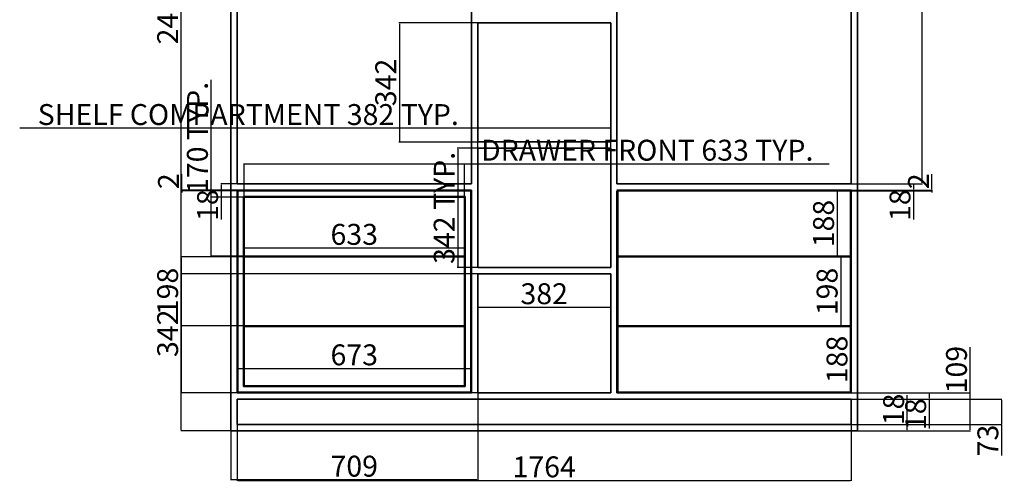
# Model space of a CAD drawing. Units: millimetres. Extents: x 222 to 5960, y 495 to 4622.
# Tile 1 of 3: x 222 to 3050, y 495 to 1826. Entities that reach past the tile are written whole.
import ezdxf

# ---------------------------------------------------------------- set-up
doc = ezdxf.new("R2010")
doc.units = ezdxf.units.MM
doc.layers.add('A-ANNO-DIMS', color=2, linetype='Continuous', lineweight=18)
doc.layers.add('A-FURN', color=7, linetype='Continuous', lineweight=35)
doc.styles.get("Standard").update_dxf_attribs({"font": 'arial.ttf'})
doc.dimstyles.new('ISO-25', dxfattribs={"dimtxt": 60, "dimasz": 2.5, "dimexe": 1.25, "dimexo": 0.625, "dimtad": 1, "dimtxsty": 'Standard', "dimcen": 2.5, "dimadec": 0, "dimazin": 0, "dimtfac": 1, "dimtmove": 0, "dimatfit": 3, "dimfxl": 1, "dimarcsym": 0})

# ---------------------------------------------------------------- blocks, each defined once
blk = doc.blocks.new('*D14')
at = {"layer": 'A-ANNO-DIMS', "color": 0, "lineweight": -2, "transparency": 16777216}
for p, q in [((2611.5, 2536.6), (2815.2, 2536.6)), ((2813.9, 2534.1), (2813.9, 1357.1)), ((2611.5, 1354.6), (2815.2, 1354.6))]:
    blk.add_line(p, q, dxfattribs=at)
at = {"layer": 'A-ANNO-DIMS', "color": 0, "transparency": 16777216}
for points in [[(2813.5, 2534.1), (2814.3, 2534.1), (2813.9, 2536.6)], [(2813.5, 1357.1), (2814.3, 1357.1), (2813.9, 1354.6)]]:
    blk.add_solid(points, dxfattribs=at)
at = {"layer": 'Defpoints', "color": 0, "transparency": 16777216}
for p in [(2610.8, 2536.6), (2610.8, 1354.6), (2813.9, 1354.6)]:
    blk.add_point(p, dxfattribs=at)
at = {"layer": 'A-ANNO-DIMS', "color": 0, "transparency": 16777216, "insert": (2782.7, 1945.6), "char_height": 60, "attachment_point": 5, "rotation": 90}
blk.add_mtext('1182', dxfattribs=at)
blk = doc.blocks.new('*D15')
at = {"layer": 'A-ANNO-DIMS', "color": 0, "lineweight": -2, "transparency": 16777216}
for p, q in [((2611.5, 1354.6), (2791, 1354.6)), ((2611.5, 1336.6), (2791, 1336.6)), ((2789.8, 1352.1), (2789.8, 1339.1)), ((2789.8, 1336.6), (2789.8, 1252.5))]:
    blk.add_line(p, q, dxfattribs=at)
at = {"layer": 'A-ANNO-DIMS', "color": 0, "transparency": 16777216}
for points in [[(2789.3, 1352.1), (2790.2, 1352.1), (2789.8, 1354.6)], [(2789.3, 1339.1), (2790.2, 1339.1), (2789.8, 1336.6)]]:
    blk.add_solid(points, dxfattribs=at)
at = {"layer": 'Defpoints', "color": 0, "transparency": 16777216}
for p in [(2610.8, 1354.6), (2610.8, 1336.6), (2789.8, 1336.6)]:
    blk.add_point(p, dxfattribs=at)
at = {"layer": 'A-ANNO-DIMS', "color": 0, "transparency": 16777216, "insert": (2758.5, 1293.3), "char_height": 60, "attachment_point": 5, "rotation": 90}
blk.add_mtext('18', dxfattribs=at)
blk = doc.blocks.new('*D24')
at = {"layer": 'A-ANNO-DIMS', "color": 0, "lineweight": -2, "transparency": 16777216}
for p, q in [((1537.2, 1816.6), (1311.5, 1816.6)), ((1312.8, 1814.1), (1312.8, 1477.1)), ((1537.2, 1474.6), (1311.5, 1474.6))]:
    blk.add_line(p, q, dxfattribs=at)
at = {"layer": 'A-ANNO-DIMS', "color": 0, "transparency": 16777216}
for points in [[(1312.4, 1814.1), (1313.2, 1814.1), (1312.8, 1816.6)], [(1312.4, 1477.1), (1313.2, 1477.1), (1312.8, 1474.6)]]:
    blk.add_solid(points, dxfattribs=at)
at = {"layer": 'Defpoints', "color": 0, "transparency": 16777216}
for p in [(1537.8, 1816.6), (1312.8, 1474.6), (1537.8, 1474.6)]:
    blk.add_point(p, dxfattribs=at)
at = {"layer": 'A-ANNO-DIMS', "color": 0, "transparency": 16777216, "insert": (1281.5, 1645.6), "char_height": 60, "attachment_point": 5, "rotation": 90}
blk.add_mtext('342', dxfattribs=at)
blk = doc.blocks.new('*D25')
at = {"layer": 'A-ANNO-DIMS', "color": 0, "lineweight": -2, "transparency": 16777216}
for p, q in [((846.2, 1354.6), (799.9, 1354.6)), ((846.2, 1336.6), (799.9, 1336.6)), ((801.1, 1352.1), (801.1, 1339.1)), ((801.1, 1336.6), (801.1, 1252.5))]:
    blk.add_line(p, q, dxfattribs=at)
at = {"layer": 'A-ANNO-DIMS', "color": 0, "transparency": 16777216}
for points in [[(800.7, 1352.1), (801.5, 1352.1), (801.1, 1354.6)], [(800.7, 1339.1), (801.5, 1339.1), (801.1, 1336.6)]]:
    blk.add_solid(points, dxfattribs=at)
at = {"layer": 'Defpoints', "color": 0, "transparency": 16777216}
for p in [(801.1, 1336.6), (846.8, 1354.6), (846.8, 1336.6)]:
    blk.add_point(p, dxfattribs=at)
at = {"layer": 'A-ANNO-DIMS', "color": 0, "transparency": 16777216, "insert": (769.9, 1293.3), "char_height": 60, "attachment_point": 5, "rotation": 90}
blk.add_mtext('18', dxfattribs=at)
blk = doc.blocks.new('*D26')
at = {"layer": 'A-ANNO-DIMS', "color": 0, "lineweight": -2, "transparency": 16777216}
for p, q in [((688.2, 1339.1), (688.2, 1382.6)), ((848.2, 1336.6), (687, 1336.6)), ((848.2, 1334.6), (687, 1334.6)), ((688.2, 1334.6), (688.2, 1336.6)), ((688.2, 1332.1), (688.2, 1329.6))]:
    blk.add_line(p, q, dxfattribs=at)
at = {"layer": 'A-ANNO-DIMS', "color": 0, "transparency": 16777216}
for points in [[(687.8, 1339.1), (688.7, 1339.1), (688.2, 1336.6)], [(687.8, 1332.1), (688.7, 1332.1), (688.2, 1334.6)]]:
    blk.add_solid(points, dxfattribs=at)
at = {"layer": 'Defpoints', "color": 0, "transparency": 16777216}
for p in [(688.2, 1336.6), (848.8, 1336.6), (848.8, 1334.6)]:
    blk.add_point(p, dxfattribs=at)
at = {"layer": 'A-ANNO-DIMS', "color": 0, "transparency": 16777216, "insert": (657.5, 1362.1), "char_height": 60, "attachment_point": 5, "rotation": 90}
blk.add_mtext('2', dxfattribs=at)
blk = doc.blocks.new('*D27')
at = {"layer": 'A-ANNO-DIMS', "color": 0, "lineweight": -2, "transparency": 16777216}
for p, q in [((2951.9, 754.6), (2951.9, 885.4)), ((2629.5, 754.6), (2953.2, 754.6)), ((2951.9, 648.1), (2951.9, 752.1)), ((2629.5, 645.6), (2953.2, 645.6))]:
    blk.add_line(p, q, dxfattribs=at)
at = {"layer": 'A-ANNO-DIMS', "color": 0, "transparency": 16777216}
for points in [[(2951.5, 752.1), (2952.3, 752.1), (2951.9, 754.6)], [(2951.5, 648.1), (2952.3, 648.1), (2951.9, 645.6)]]:
    blk.add_solid(points, dxfattribs=at)
at = {"layer": 'Defpoints', "color": 0, "transparency": 16777216}
for p in [(2628.8, 754.6), (2951.9, 754.6), (2628.8, 645.6)]:
    blk.add_point(p, dxfattribs=at)
at = {"layer": 'A-ANNO-DIMS', "color": 0, "transparency": 16777216, "insert": (2920.7, 821.3), "char_height": 60, "attachment_point": 5, "rotation": 90}
blk.add_mtext('109', dxfattribs=at)
blk = doc.blocks.new('*D28')
at = {"layer": 'A-ANNO-DIMS', "color": 0, "lineweight": -2, "transparency": 16777216}
for p, q in [((2611.5, 754.6), (2835.9, 754.6)), ((2611.5, 736.6), (2835.9, 736.6)), ((2834.6, 752.1), (2834.6, 739.1)), ((2834.6, 736.6), (2834.6, 652.5))]:
    blk.add_line(p, q, dxfattribs=at)
at = {"layer": 'A-ANNO-DIMS', "color": 0, "transparency": 16777216}
for points in [[(2834.2, 752.1), (2835, 752.1), (2834.6, 754.6)], [(2834.2, 739.1), (2835, 739.1), (2834.6, 736.6)]]:
    blk.add_solid(points, dxfattribs=at)
at = {"layer": 'Defpoints', "color": 0, "transparency": 16777216}
for p in [(2610.8, 754.6), (2610.8, 736.6), (2834.6, 736.6)]:
    blk.add_point(p, dxfattribs=at)
at = {"layer": 'A-ANNO-DIMS', "color": 0, "transparency": 16777216, "insert": (2803.4, 693.3), "char_height": 60, "attachment_point": 5, "rotation": 90}
blk.add_mtext('18', dxfattribs=at)
blk = doc.blocks.new('*D29')
at = {"layer": 'A-ANNO-DIMS', "color": 0, "lineweight": -2, "transparency": 16777216}
for p, q in [((2611.5, 736.6), (3043.5, 736.6)), ((3042.2, 734.1), (3042.2, 666.1)), ((2611.5, 663.6), (3043.5, 663.6)), ((3042.2, 663.6), (3042.2, 574.4))]:
    blk.add_line(p, q, dxfattribs=at)
at = {"layer": 'A-ANNO-DIMS', "color": 0, "transparency": 16777216}
for points in [[(3041.8, 734.1), (3042.6, 734.1), (3042.2, 736.6)], [(3041.8, 666.1), (3042.6, 666.1), (3042.2, 663.6)]]:
    blk.add_solid(points, dxfattribs=at)
at = {"layer": 'Defpoints', "color": 0, "transparency": 16777216}
for p in [(2610.8, 736.6), (2610.8, 663.6), (3042.2, 663.6)]:
    blk.add_point(p, dxfattribs=at)
at = {"layer": 'A-ANNO-DIMS', "color": 0, "transparency": 16777216, "insert": (3010.9, 617.8), "char_height": 60, "attachment_point": 5, "rotation": 90}
blk.add_mtext('73', dxfattribs=at)
blk = doc.blocks.new('*D30')
at = {"layer": 'A-ANNO-DIMS', "color": 0, "lineweight": -2, "transparency": 16777216}
for p, q in [((2842.3, 1339.1), (2842.3, 1382.6)), ((2609.5, 1336.6), (2843.6, 1336.6)), ((2609.5, 1334.6), (2843.6, 1334.6)), ((2842.3, 1334.6), (2842.3, 1336.6)), ((2842.3, 1332.1), (2842.3, 1329.6))]:
    blk.add_line(p, q, dxfattribs=at)
at = {"layer": 'A-ANNO-DIMS', "color": 0, "transparency": 16777216}
for points in [[(2841.9, 1339.1), (2842.7, 1339.1), (2842.3, 1336.6)], [(2841.9, 1332.1), (2842.7, 1332.1), (2842.3, 1334.6)]]:
    blk.add_solid(points, dxfattribs=at)
at = {"layer": 'Defpoints', "color": 0, "transparency": 16777216}
for p in [(2608.8, 1336.6), (2608.8, 1334.6), (2842.3, 1336.6)]:
    blk.add_point(p, dxfattribs=at)
at = {"layer": 'A-ANNO-DIMS', "color": 0, "transparency": 16777216, "insert": (2811.6, 1362.1), "char_height": 60, "attachment_point": 5, "rotation": 90}
blk.add_mtext('2', dxfattribs=at)
blk = doc.blocks.new('*D31')
at = {"layer": 'A-ANNO-DIMS', "color": 0, "lineweight": -2, "transparency": 16777216}
for p, q in [((2608.2, 1334.6), (2569, 1334.6)), ((2570.2, 1332.1), (2570.2, 1149.1)), ((2608.2, 1146.6), (2569, 1146.6))]:
    blk.add_line(p, q, dxfattribs=at)
at = {"layer": 'A-ANNO-DIMS', "color": 0, "transparency": 16777216}
for points in [[(2569.8, 1332.1), (2570.7, 1332.1), (2570.2, 1334.6)], [(2569.8, 1149.1), (2570.7, 1149.1), (2570.2, 1146.6)]]:
    blk.add_solid(points, dxfattribs=at)
at = {"layer": 'Defpoints', "color": 0, "transparency": 16777216}
for p in [(2608.8, 1334.6), (2570.2, 1146.6), (2608.8, 1146.6)]:
    blk.add_point(p, dxfattribs=at)
at = {"layer": 'A-ANNO-DIMS', "color": 0, "transparency": 16777216, "insert": (2539, 1240.6), "char_height": 60, "attachment_point": 5, "rotation": 90}
blk.add_mtext('188', dxfattribs=at)
blk = doc.blocks.new('*D32')
at = {"layer": 'A-ANNO-DIMS', "color": 0, "lineweight": -2, "transparency": 16777216}
for p, q in [((2608.2, 1144.6), (2579.2, 1144.6)), ((2580.4, 1142.1), (2580.4, 949.1)), ((2608.2, 946.6), (2579.2, 946.6))]:
    blk.add_line(p, q, dxfattribs=at)
at = {"layer": 'A-ANNO-DIMS', "color": 0, "transparency": 16777216}
for points in [[(2580, 1142.1), (2580.9, 1142.1), (2580.4, 1144.6)], [(2580, 949.1), (2580.9, 949.1), (2580.4, 946.6)]]:
    blk.add_solid(points, dxfattribs=at)
at = {"layer": 'Defpoints', "color": 0, "transparency": 16777216}
for p in [(2608.8, 1144.6), (2580.4, 946.6), (2608.8, 946.6)]:
    blk.add_point(p, dxfattribs=at)
at = {"layer": 'A-ANNO-DIMS', "color": 0, "transparency": 16777216, "insert": (2549.2, 1045.6), "char_height": 60, "attachment_point": 5, "rotation": 90}
blk.add_mtext('198', dxfattribs=at)
blk = doc.blocks.new('*D33')
at = {"layer": 'A-ANNO-DIMS', "color": 0, "lineweight": -2, "transparency": 16777216}
for p, q in [((2608.8, 942.1), (2608.8, 759.1)), ((2609.5, 944.6), (2610.1, 944.6)), ((2609.5, 756.6), (2610.1, 756.6))]:
    blk.add_line(p, q, dxfattribs=at)
at = {"layer": 'A-ANNO-DIMS', "color": 0, "transparency": 16777216}
for points in [[(2608.4, 942.1), (2609.3, 942.1), (2608.8, 944.6)], [(2608.4, 759.1), (2609.3, 759.1), (2608.8, 756.6)]]:
    blk.add_solid(points, dxfattribs=at)
at = {"layer": 'Defpoints', "color": 0, "transparency": 16777216}
for p in [(2608.8, 944.6), (2608.8, 756.6), (2608.8, 756.6)]:
    blk.add_point(p, dxfattribs=at)
at = {"layer": 'A-ANNO-DIMS', "color": 0, "transparency": 16777216, "insert": (2577.6, 850.6), "char_height": 60, "attachment_point": 5, "rotation": 90}
blk.add_mtext('188', dxfattribs=at)
blk = doc.blocks.new('*D34')
at = {"layer": 'A-ANNO-DIMS', "color": 0, "lineweight": -2, "transparency": 16777216}
for p, q in [((866.8, 1145.3), (866.8, 1171.7)), ((869.3, 1170.5), (1497.3, 1170.5)), ((1499.8, 1145.3), (1499.8, 1171.7))]:
    blk.add_line(p, q, dxfattribs=at)
at = {"layer": 'A-ANNO-DIMS', "color": 0, "transparency": 16777216}
for points in [[(869.3, 1170.9), (869.3, 1170), (866.8, 1170.5)], [(1497.3, 1170.9), (1497.3, 1170), (1499.8, 1170.5)]]:
    blk.add_solid(points, dxfattribs=at)
at = {"layer": 'Defpoints', "color": 0, "transparency": 16777216}
for p in [(1499.8, 1170.5), (866.8, 1144.6), (1499.8, 1144.6)]:
    blk.add_point(p, dxfattribs=at)
at = {"layer": 'A-ANNO-DIMS', "color": 0, "transparency": 16777216, "insert": (1183.3, 1201.7), "char_height": 60, "attachment_point": 5}
blk.add_mtext('633', dxfattribs=at)
blk = doc.blocks.new('*D35')
at = {"layer": 'A-ANNO-DIMS', "color": 0, "lineweight": -2, "transparency": 16777216}
for p, q in [((828.8, 754), (828.8, 503.9)), ((1537.8, 754), (1537.8, 503.9)), ((1535.3, 505.1), (831.3, 505.1))]:
    blk.add_line(p, q, dxfattribs=at)
at = {"layer": 'A-ANNO-DIMS', "color": 0, "transparency": 16777216}
for points in [[(831.3, 505.6), (831.3, 504.7), (828.8, 505.1)], [(1535.3, 505.6), (1535.3, 504.7), (1537.8, 505.1)]]:
    blk.add_solid(points, dxfattribs=at)
at = {"layer": 'Defpoints', "color": 0, "transparency": 16777216}
for p in [(828.8, 754.6), (1537.8, 754.6), (828.8, 505.1)]:
    blk.add_point(p, dxfattribs=at)
at = {"layer": 'A-ANNO-DIMS', "color": 0, "transparency": 16777216, "insert": (1183.3, 536.4), "char_height": 60, "attachment_point": 5}
blk.add_mtext('709', dxfattribs=at)
blk = doc.blocks.new('*D36')
at = {"layer": 'A-ANNO-DIMS', "color": 0, "lineweight": -2, "transparency": 16777216}
for p, q in [((846.8, 755.3), (846.8, 825.9)), ((849.3, 824.6), (1517.3, 824.6)), ((1519.8, 755.3), (1519.8, 825.9))]:
    blk.add_line(p, q, dxfattribs=at)
at = {"layer": 'A-ANNO-DIMS', "color": 0, "transparency": 16777216}
for points in [[(849.3, 825), (849.3, 824.2), (846.8, 824.6)], [(1517.3, 825), (1517.3, 824.2), (1519.8, 824.6)]]:
    blk.add_solid(points, dxfattribs=at)
at = {"layer": 'Defpoints', "color": 0, "transparency": 16777216}
for p in [(1519.8, 824.6), (846.8, 754.6), (1519.8, 754.6)]:
    blk.add_point(p, dxfattribs=at)
at = {"layer": 'A-ANNO-DIMS', "color": 0, "transparency": 16777216, "insert": (1183.3, 855.9), "char_height": 60, "attachment_point": 5}
blk.add_mtext('673', dxfattribs=at)
blk = doc.blocks.new('*D37')
at = {"layer": 'A-ANNO-DIMS', "color": 0, "lineweight": -2, "transparency": 16777216}
for p, q in [((1537.8, 1096), (1537.8, 998.9)), ((1919.8, 1096), (1919.8, 998.9)), ((1540.3, 1000.2), (1917.3, 1000.2))]:
    blk.add_line(p, q, dxfattribs=at)
at = {"layer": 'A-ANNO-DIMS', "color": 0, "transparency": 16777216}
for points in [[(1540.3, 1000.6), (1540.3, 999.7), (1537.8, 1000.2)], [(1917.3, 1000.6), (1917.3, 999.7), (1919.8, 1000.2)]]:
    blk.add_solid(points, dxfattribs=at)
at = {"layer": 'Defpoints', "color": 0, "transparency": 16777216}
for p in [(1537.8, 1096.6), (1919.8, 1096.6), (1919.8, 1000.2)]:
    blk.add_point(p, dxfattribs=at)
at = {"layer": 'A-ANNO-DIMS', "color": 0, "transparency": 16777216, "insert": (1728.8, 1031.4), "char_height": 60, "attachment_point": 5}
blk.add_mtext('382', dxfattribs=at)
blk = doc.blocks.new('SHELF-COMPARTMENT')
for p, q in [((0, 342), (0, 0)), ((0, 342), (382, 342)), ((382, 342), (382, 0)), ((0, 0), (382, 0))]:
    blk.add_line(p, q)
blk = doc.blocks.new('DRAWER-FRONT')
for p, q in [((0, 170), (0, 0)), ((0, 170), (633, 170)), ((633, 170), (633, 0)), ((0, 0), (633, 0))]:
    blk.add_line(p, q)
blk = doc.blocks.new('*D55')
at = {"layer": 'A-ANNO-DIMS', "color": 0, "lineweight": -2, "transparency": 16777216}
for p, q in [((1537.8, 1513.9), (222.4, 1513.9)), ((1537.8, 1457.3), (1537.8, 1515.2)), ((1917.3, 1513.9), (1540.3, 1513.9)), ((1919.8, 1457.3), (1919.8, 1515.2))]:
    blk.add_line(p, q, dxfattribs=at)
at = {"layer": 'A-ANNO-DIMS', "color": 0, "transparency": 16777216}
for points in [[(1540.3, 1514.4), (1540.3, 1513.5), (1537.8, 1513.9)], [(1917.3, 1514.4), (1917.3, 1513.5), (1919.8, 1513.9)]]:
    blk.add_solid(points, dxfattribs=at)
at = {"layer": 'Defpoints', "color": 0, "transparency": 16777216}
for p in [(1537.8, 1513.9), (1537.8, 1456.6), (1919.8, 1456.6)]:
    blk.add_point(p, dxfattribs=at)
at = {"layer": 'A-ANNO-DIMS', "color": 0, "transparency": 16777216, "insert": (878.9, 1545.6), "char_height": 60, "attachment_point": 5}
blk.add_mtext('SHELF COMPARTMENT 382 TYP.', dxfattribs=at)
blk = doc.blocks.new('*D56')
at = {"layer": 'A-ANNO-DIMS', "color": 0, "lineweight": -2, "transparency": 16777216}
for p, q in [((1537.2, 1456.6), (1479.3, 1456.6)), ((1480.5, 1454.1), (1480.5, 1117.1)), ((1537.2, 1114.6), (1479.3, 1114.6))]:
    blk.add_line(p, q, dxfattribs=at)
at = {"layer": 'A-ANNO-DIMS', "color": 0, "transparency": 16777216}
for points in [[(1480.1, 1454.1), (1481, 1454.1), (1480.5, 1456.6)], [(1480.1, 1117.1), (1481, 1117.1), (1480.5, 1114.6)]]:
    blk.add_solid(points, dxfattribs=at)
at = {"layer": 'Defpoints', "color": 0, "transparency": 16777216}
for p in [(1537.8, 1456.6), (1480.5, 1114.6), (1537.8, 1114.6)]:
    blk.add_point(p, dxfattribs=at)
at = {"layer": 'A-ANNO-DIMS', "color": 0, "transparency": 16777216, "insert": (1449.3, 1285.6), "char_height": 60, "attachment_point": 5, "rotation": 90}
blk.add_mtext('342 TYP.', dxfattribs=at)
blk = doc.blocks.new('*D57')
at = {"layer": 'A-ANNO-DIMS', "color": 0, "lineweight": -2, "transparency": 16777216}
for p, q in [((866.8, 1317.3), (866.8, 1412.8)), ((869.3, 1411.6), (1497.3, 1411.6)), ((1499.8, 1317.3), (1499.8, 1412.8)), ((1499.8, 1411.6), (2547, 1411.6))]:
    blk.add_line(p, q, dxfattribs=at)
at = {"layer": 'A-ANNO-DIMS', "color": 0, "transparency": 16777216}
for points in [[(869.3, 1412), (869.3, 1411.2), (866.8, 1411.6)], [(1497.3, 1412), (1497.3, 1411.2), (1499.8, 1411.6)]]:
    blk.add_solid(points, dxfattribs=at)
at = {"layer": 'Defpoints', "color": 0, "transparency": 16777216}
for p in [(1499.8, 1411.6), (866.8, 1316.6), (1499.8, 1316.6)]:
    blk.add_point(p, dxfattribs=at)
at = {"layer": 'A-ANNO-DIMS', "color": 0, "transparency": 16777216, "insert": (2024.7, 1443.3), "char_height": 60, "attachment_point": 5}
blk.add_mtext('DRAWER FRONT 633 TYP.', dxfattribs=at)
blk = doc.blocks.new('*D58')
at = {"layer": 'A-ANNO-DIMS', "color": 0, "lineweight": -2, "transparency": 16777216}
for p, q in [((771.9, 1316.6), (771.9, 1653.4)), ((866.2, 1316.6), (770.6, 1316.6)), ((771.9, 1149.1), (771.9, 1314.1)), ((866.2, 1146.6), (770.6, 1146.6))]:
    blk.add_line(p, q, dxfattribs=at)
at = {"layer": 'A-ANNO-DIMS', "color": 0, "transparency": 16777216}
for points in [[(771.5, 1314.1), (772.3, 1314.1), (771.9, 1316.6)], [(771.5, 1149.1), (772.3, 1149.1), (771.9, 1146.6)]]:
    blk.add_solid(points, dxfattribs=at)
at = {"layer": 'Defpoints', "color": 0, "transparency": 16777216}
for p in [(771.9, 1316.6), (866.8, 1316.6), (866.8, 1146.6)]:
    blk.add_point(p, dxfattribs=at)
at = {"layer": 'A-ANNO-DIMS', "color": 0, "transparency": 16777216, "insert": (740.6, 1486.3), "char_height": 60, "attachment_point": 5, "rotation": 90}
blk.add_mtext('170 TYP.', dxfattribs=at)
blk = doc.blocks.new('*D59')
at = {"layer": 'A-ANNO-DIMS', "color": 0, "lineweight": -2, "transparency": 16777216}
for p, q in [((828.2, 3045.6), (685.1, 3045.6)), ((686.3, 648.1), (686.3, 3043.1)), ((828.2, 645.6), (685.1, 645.6))]:
    blk.add_line(p, q, dxfattribs=at)
at = {"layer": 'A-ANNO-DIMS', "color": 0, "transparency": 16777216}
for points in [[(685.9, 3043.1), (686.8, 3043.1), (686.3, 3045.6)], [(685.9, 648.1), (686.8, 648.1), (686.3, 645.6)]]:
    blk.add_solid(points, dxfattribs=at)
at = {"layer": 'Defpoints', "color": 0, "transparency": 16777216}
for p in [(686.3, 3045.6), (828.8, 3045.6), (828.8, 645.6)]:
    blk.add_point(p, dxfattribs=at)
at = {"layer": 'A-ANNO-DIMS', "color": 0, "transparency": 16777216, "insert": (655.1, 1845.6), "char_height": 60, "attachment_point": 5, "rotation": 90}
blk.add_mtext('2400', dxfattribs=at)
blk = doc.blocks.new('*D60')
at = {"layer": 'A-ANNO-DIMS', "color": 0, "lineweight": -2, "transparency": 16777216}
for p, q in [((866.2, 1144.6), (685.1, 1144.6)), ((686.3, 1142.1), (686.3, 949.1)), ((866.2, 946.6), (685.1, 946.6))]:
    blk.add_line(p, q, dxfattribs=at)
at = {"layer": 'A-ANNO-DIMS', "color": 0, "transparency": 16777216}
for points in [[(685.9, 1142.1), (686.8, 1142.1), (686.3, 1144.6)], [(685.9, 949.1), (686.8, 949.1), (686.3, 946.6)]]:
    blk.add_solid(points, dxfattribs=at)
at = {"layer": 'Defpoints', "color": 0, "transparency": 16777216}
for p in [(866.8, 1144.6), (686.3, 946.6), (866.8, 946.6)]:
    blk.add_point(p, dxfattribs=at)
at = {"layer": 'A-ANNO-DIMS', "color": 0, "transparency": 16777216, "insert": (655.1, 1045.6), "char_height": 60, "attachment_point": 5, "rotation": 90}
blk.add_mtext('198', dxfattribs=at)
blk = doc.blocks.new('*D61')
at = {"layer": 'A-ANNO-DIMS', "color": 0, "lineweight": -2, "transparency": 16777216}
for p, q in [((1537.2, 1096.6), (685.1, 1096.6)), ((686.3, 1094.1), (686.3, 757.1)), ((1537.2, 754.6), (685.1, 754.6))]:
    blk.add_line(p, q, dxfattribs=at)
at = {"layer": 'A-ANNO-DIMS', "color": 0, "transparency": 16777216}
for points in [[(685.9, 1094.1), (686.8, 1094.1), (686.3, 1096.6)], [(685.9, 757.1), (686.8, 757.1), (686.3, 754.6)]]:
    blk.add_solid(points, dxfattribs=at)
at = {"layer": 'Defpoints', "color": 0, "transparency": 16777216}
for p in [(1537.8, 1096.6), (686.3, 754.6), (1537.8, 754.6)]:
    blk.add_point(p, dxfattribs=at)
at = {"layer": 'A-ANNO-DIMS', "color": 0, "transparency": 16777216, "insert": (655.1, 925.6), "char_height": 60, "attachment_point": 5, "rotation": 90}
blk.add_mtext('342', dxfattribs=at)
blk = doc.blocks.new('*D62')
at = {"layer": 'A-ANNO-DIMS', "color": 0, "lineweight": -2, "transparency": 16777216}
for p, q in [((846.8, 663), (846.8, 501.9)), ((2610.8, 663), (2610.8, 501.9)), ((849.3, 503.1), (2608.3, 503.1))]:
    blk.add_line(p, q, dxfattribs=at)
at = {"layer": 'A-ANNO-DIMS', "color": 0, "transparency": 16777216}
for points in [[(849.3, 503.6), (849.3, 502.7), (846.8, 503.1)], [(2608.3, 503.6), (2608.3, 502.7), (2610.8, 503.1)]]:
    blk.add_solid(points, dxfattribs=at)
at = {"layer": 'Defpoints', "color": 0, "transparency": 16777216}
for p in [(846.8, 663.6), (2610.8, 663.6), (2610.8, 503.1)]:
    blk.add_point(p, dxfattribs=at)
at = {"layer": 'A-ANNO-DIMS', "color": 0, "transparency": 16777216, "insert": (1728.8, 534.4), "char_height": 60, "attachment_point": 5}
blk.add_mtext('1764', dxfattribs=at)
blk = doc.blocks.new('*D63')
at = {"layer": 'A-ANNO-DIMS', "color": 0, "lineweight": -2, "transparency": 16777216}
for p, q in [((2771.3, 663.6), (2771.3, 747.8)), ((2611.5, 663.6), (2772.6, 663.6)), ((2771.3, 648.1), (2771.3, 661.1)), ((2629.5, 645.6), (2772.6, 645.6))]:
    blk.add_line(p, q, dxfattribs=at)
at = {"layer": 'A-ANNO-DIMS', "color": 0, "transparency": 16777216}
for points in [[(2770.9, 661.1), (2771.8, 661.1), (2771.3, 663.6)], [(2770.9, 648.1), (2771.8, 648.1), (2771.3, 645.6)]]:
    blk.add_solid(points, dxfattribs=at)
at = {"layer": 'Defpoints', "color": 0, "transparency": 16777216}
for p in [(2610.8, 663.6), (2771.3, 663.6), (2628.8, 645.6)]:
    blk.add_point(p, dxfattribs=at)
at = {"layer": 'A-ANNO-DIMS', "color": 0, "transparency": 16777216, "insert": (2740.1, 707), "char_height": 60, "attachment_point": 5, "rotation": 90}
blk.add_mtext('18', dxfattribs=at)

msp = doc.modelspace()

# ---------------------------------------------------------------- linework, layer by layer
at = {"layer": 'A-FURN'}
for p, q in [((828.845, 3045.641), (828.845, 645.641)), ((2628.845, 645.641), (2628.845, 3045.641)), ((828.845, 2545.641), (828.845, 645.641)), ((846.845, 2545.641), (846.845, 1354.641)), ((1519.845, 2536.641), (1519.845, 1354.641)), ((1937.845, 2536.641), (1937.845, 1354.641)), ((2610.845, 1354.641), (2610.845, 2536.641)), ((846.845, 1354.641), (1519.845, 1354.641)), ((846.845, 1336.641), (1519.845, 1336.641)), ((846.845, 1336.641), (846.845, 754.641)), ((848.845, 1334.641), (848.845, 1144.641)), ((848.845, 1334.641), (1517.845, 1334.641)), ((1517.845, 1334.641), (1517.845, 1144.641)), ((1519.845, 1336.641), (1519.845, 754.641)), ((1937.845, 1354.641), (2610.845, 1354.641)), ((1937.845, 1336.641), (2610.845, 1336.641)), ((1937.845, 1334.641), (2608.845, 1334.641)), ((1937.845, 1334.641), (1937.845, 754.641)), ((1939.845, 1334.641), (1939.845, 1146.641)), ((2608.845, 1146.641), (2608.845, 1334.641)), ((2610.845, 944.641), (2610.845, 1336.641)), ((864.845, 1318.641), (1501.845, 1318.641)), ((864.845, 1318.641), (864.845, 1144.641)), ((1501.845, 1318.641), (1501.845, 1144.641)), ((848.845, 1144.641), (848.845, 944.641)), ((864.845, 1144.641), (864.845, 944.641)), ((866.845, 1144.641), (866.845, 946.641)), ((866.845, 1144.641), (1499.845, 1144.641)), ((1499.845, 1144.641), (1499.845, 946.641)), ((1501.845, 1144.641), (1501.845, 772.641)), ((1517.845, 1144.641), (1517.845, 944.641)), ((1939.845, 1146.641), (2608.845, 1146.641)), ((1939.845, 1144.641), (2608.845, 1144.641)), ((1939.845, 1144.641), (1939.845, 946.641)), ((2608.845, 946.641), (2608.845, 1144.641)), ((848.845, 944.641), (848.845, 756.641)), ((864.845, 944.641), (864.845, 772.641)), ((866.845, 946.641), (1499.845, 946.641)), ((1517.845, 944.641), (1517.845, 756.641)), ((1939.845, 946.641), (2608.845, 946.641)), ((1939.845, 944.641), (2608.845, 944.641)), ((1939.845, 944.641), (1939.845, 756.641)), ((2608.845, 756.641), (2608.845, 944.641)), ((2610.845, 754.641), (2610.845, 944.641)), ((864.845, 772.641), (1501.845, 772.641)), ((846.845, 754.641), (1519.845, 754.641)), ((846.845, 736.641), (2610.845, 736.641)), ((846.845, 736.641), (846.845, 663.641)), ((848.845, 756.641), (1517.845, 756.641)), ((1937.845, 754.641), (2610.845, 754.641)), ((1939.845, 756.641), (2608.845, 756.641)), ((2610.845, 663.641), (2610.845, 736.641)), ((846.845, 663.641), (2610.845, 663.641)), ((828.845, 645.641), (2628.845, 645.641))]:
    msp.add_line(p, q, dxfattribs=at)

# ---------------------------------------------------------------- block references
at = {"layer": 'A-FURN', "rotation": 180}
for p in [(1919.845, 1816.641), (1919.845, 1456.641)]:
    msp.add_blockref('SHELF-COMPARTMENT', p, dxfattribs=at)
at = {"layer": 'A-FURN'}
for name, p in [('DRAWER-FRONT', (866.845, 1146.641)), ('SHELF-COMPARTMENT', (1537.845, 754.641)), ('DRAWER-FRONT', (866.845, 774.641))]:
    msp.add_blockref(name, p, dxfattribs=at)

# ---------------------------------------------------------------- dimensions: what is measured, and where the dimension line sits
at = {"layer": 'A-ANNO-DIMS'}
for base, p1, p2, override, picture, middle in [((686.345, 3045.641), (828.845, 645.641), (828.845, 3045.641), {"dimdec": 0, "dimlfac": 1, "dimrnd": 0, "dimzin": 0, "dimdsep": 46, "dimlunit": 2}, '*D59', (655.085, 1845.641)), ((2813.931, 1354.641), (2610.845, 2536.641), (2610.845, 1354.641), {"dimclrd": 0, "dimclre": 0, "dimclrt": 0}, '*D14', (2782.672, 1945.641)), ((1312.77, 1474.641), (1537.845, 1816.641), (1537.845, 1474.641), {"dimclrd": 0, "dimclre": 0, "dimclrt": 0}, '*D24', (1281.49, 1645.641)), ((688.246, 1336.641), (848.845, 1334.641), (848.845, 1336.641), {"dimclrd": 0, "dimclre": 0, "dimclrt": 0}, '*D26', (657.498, 1362.136)), ((2842.33, 1336.641), (2608.845, 1334.641), (2608.845, 1336.641), {"dimclrd": 0, "dimclre": 0, "dimclrt": 0}, '*D30', (2811.582, 1362.136)), ((801.11, 1336.641), (846.845, 1354.641), (846.845, 1336.641), {"dimclrd": 0, "dimclre": 0, "dimclrt": 0}, '*D25', (769.85, 1293.305)), ((2570.246, 1146.641), (2608.845, 1334.641), (2608.845, 1146.641), {"dimclrd": 0, "dimclre": 0, "dimclrt": 0}, '*D31', (2538.987, 1240.641)), ((2789.754, 1336.641), (2610.845, 1354.641), (2610.845, 1336.641), {"dimclrd": 0, "dimclre": 0, "dimclrt": 0}, '*D15', (2758.494, 1293.305)), ((686.345, 946.641), (866.845, 1144.641), (866.845, 946.641), {"dimdec": 0, "dimlfac": 1, "dimrnd": 0, "dimzin": 0, "dimdsep": 46, "dimlunit": 2}, '*D60', (655.085, 1045.641)), ((2580.449, 946.641), (2608.845, 1144.641), (2608.845, 946.641), {"dimclrd": 0, "dimclre": 0, "dimclrt": 0}, '*D32', (2549.189, 1045.641)), ((686.345, 754.641), (1537.845, 1096.641), (1537.845, 754.641), {"dimdec": 0, "dimlfac": 1, "dimrnd": 0, "dimzin": 0, "dimdsep": 46, "dimlunit": 2}, '*D61', (655.065, 925.641)), ((2608.845, 756.641), (2608.845, 944.641), (2608.845, 756.641), {"dimclrd": 0, "dimclre": 0, "dimclrt": 0}, '*D33', (2577.585, 850.641)), ((2951.918, 754.641), (2628.845, 645.641), (2628.845, 754.641), {"dimclrd": 0, "dimclre": 0, "dimclrt": 0}, '*D27', (2920.659, 821.286)), ((2834.631, 736.641), (2610.845, 754.641), (2610.845, 736.641), {"dimclrd": 0, "dimclre": 0, "dimclrt": 0}, '*D28', (2803.372, 693.305)), ((2771.345, 663.641), (2628.845, 645.641), (2610.845, 663.641), {"dimdec": 0, "dimlfac": 1, "dimrnd": 0, "dimzin": 0, "dimdsep": 46, "dimlunit": 2}, '*D63', (2740.085, 706.977)), ((3042.224, 663.641), (2610.845, 736.641), (2610.845, 663.641), {"dimclrd": 0, "dimclre": 0, "dimclrt": 0}, '*D29', (3010.944, 617.787))]:
    dim = msp.add_linear_dim(base=base, p1=p1, p2=p2, angle=90, dimstyle='ISO-25', override=override, dxfattribs=at)
    dim.commit()
    dim.dimension.update_dxf_attribs({"geometry": picture, "text_midpoint": middle})
for base, p1, p2, angle, text, picture, middle in [((1537.845, 1513.941), (1919.845, 1456.641), (1537.845, 1456.641), 180, 'SHELF COMPARTMENT <> TYP.', '*D55', (878.874, 1545.63)), ((771.895, 1316.641), (866.845, 1146.641), (866.845, 1316.641), 90, '<> TYP.', '*D58', (740.635, 1486.28)), ((1480.545, 1114.641), (1537.845, 1456.641), (1537.845, 1114.641), 270, '<> TYP.', '*D56', (1449.265, 1285.641))]:
    dim = msp.add_linear_dim(base=base, p1=p1, p2=p2, angle=angle, text=text, dimstyle='ISO-25', override={"dimdec": 0, "dimrnd": 0, "dimzin": 0, "dimlunit": 2}, dxfattribs=at)
    dim.commit()
    dim.dimension.update_dxf_attribs({"geometry": picture, "text_midpoint": middle})
dim = msp.add_linear_dim(base=(1499.845, 1411.591), p1=(866.845, 1316.641), p2=(1499.845, 1316.641), text='DRAWER FRONT <> TYP.', dimstyle='ISO-25', override={"dimdec": 0, "dimrnd": 0, "dimzin": 0, "dimlunit": 2}, dxfattribs=at)
dim.commit()
dim.dimension.update_dxf_attribs({"geometry": '*D57', "text_midpoint": (2024.696, 1443.28)})
for base, p1, p2, override, picture, middle in [((1499.845, 1170.462), (866.845, 1144.641), (1499.845, 1144.641), {"dimclrd": 0, "dimclre": 0, "dimclrt": 0}, '*D34', (1183.345, 1201.742)), ((1919.845, 1000.166), (1537.845, 1096.641), (1919.845, 1096.641), {"dimclrd": 0, "dimclre": 0, "dimclrt": 0}, '*D37', (1728.845, 1031.446)), ((1519.845, 824.604), (846.845, 754.641), (1519.845, 754.641), {"dimclrd": 0, "dimclre": 0, "dimclrt": 0}, '*D36', (1183.345, 855.884)), ((828.845, 505.148), (1537.845, 754.641), (828.845, 754.641), {"dimclrd": 0, "dimclre": 0, "dimclrt": 0}, '*D35', (1183.345, 536.408)), ((2610.845, 503.141), (846.845, 663.641), (2610.845, 663.641), {"dimdec": 0, "dimlfac": 1, "dimrnd": 0, "dimzin": 0, "dimdsep": 46, "dimlunit": 2}, '*D62', (1728.845, 534.4))]:
    dim = msp.add_linear_dim(base=base, p1=p1, p2=p2, dimstyle='ISO-25', override=override, dxfattribs=at)
    dim.commit()
    dim.dimension.update_dxf_attribs({"geometry": picture, "text_midpoint": middle})

doc.saveas('drawing.dxf')
